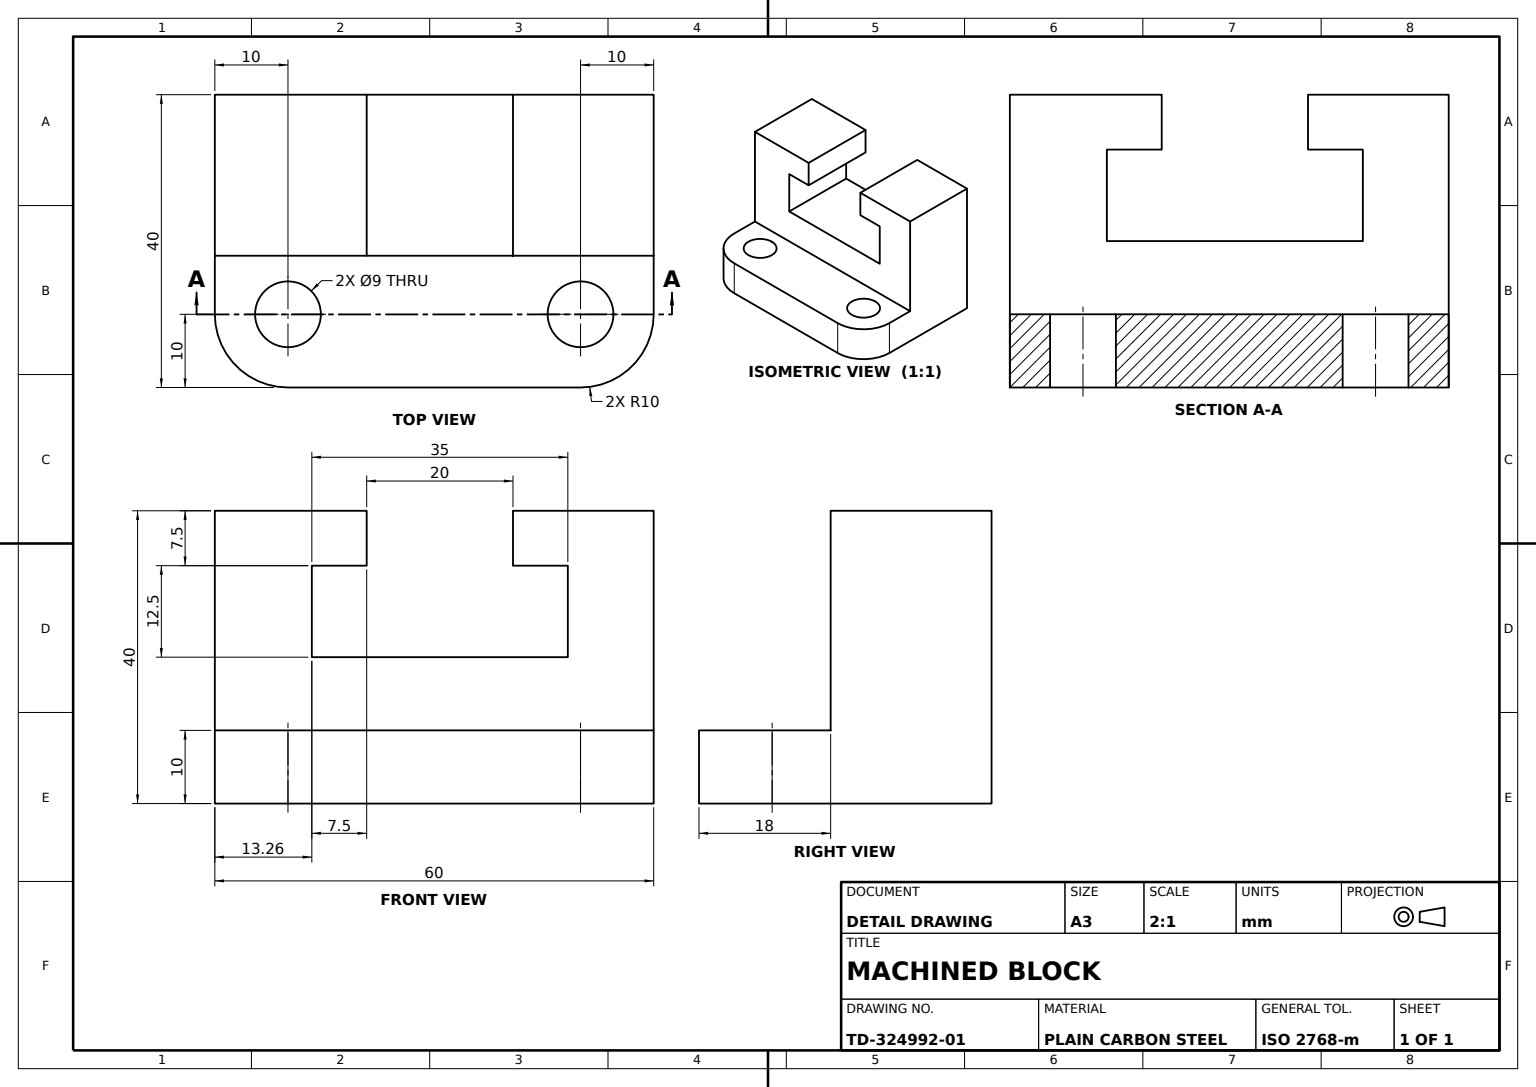
SolidWorks part; units mm, degrees
material "Plain Carbon Steel"
ref_plane "Front Plane" through (0, 0, 0) normal (0, 0, 1) x (1, 0, 0)
ref_plane "Top Plane" through (0, 0, 0) normal (0, 1, 0) x (1, 0, 0)
ref_plane "Right Plane" through (0, 0, 0) normal (1, 0, 0) x (0, 0, -1)
sketch "U-Bracket Profile Sketch" plane through (0, 0, 0) normal (0, 0, 1) x (1, 0, 0)
  line L0 (0, 0) -> (60, 0)
  line L1 (60, 0) -> (60, 40)
  line L2 (60, 40) -> (40.7619, 40)
  line L3 (40.7619, 40) -> (40.7619, 32.5)
  line L4 (40.7619, 32.5) -> (48.2619, 32.5)
  line L5 (48.2619, 32.5) -> (48.2619, 20)
  line L6 (48.2619, 20) -> (13.2619, 20)
  line L7 (13.2619, 20) -> (13.2619, 32.5)
  line L8 (20.7619, 32.5) -> (20.7619, 40)
  line L9 (20.7619, 40) -> (0, 40)
  line L10 (0, 40) -> (0, 0)
  line L11 (13.2619, 32.5) -> (20.7619, 32.5)
  point P12 (40.7619, 36.25)
  dimension "D1" = 60
  dimension "D2" = 40
  dimension "D3" = 20
  dimension "D4" = 35
  dimension "D5" = 7.5
  dimension "D6" = 7.5
  dimension "D7" = 12.5
  dimension "D8" = 12.5
  dimension "D9" = 7.5
  dimension "D10" = 13.2619
extrude "U-Bracket Body" add sketch "U-Bracket Profile Sketch" along normal blind 22
sketch "Base Plate Sketch" plane through (0, 0, 0) normal (0, -1, 0) x (1, 0, 0)
  line L0 (0, 22) -> (0, 30)
  line L1 (10, 40) -> (50, 40)
  line L2 (60, 30) -> (60, 22)
  line L7 (0, 0) -> (60, 0)
  line L8 (60, 0) -> (60, 22)
  line L9 (60, 22) -> (0, 22)
  line L10 (0, 22) -> (0, 0)
  line L11 (0, 0) -> (60, 0)
  line L12 (60, 0) -> (60, 22)
  line L14 (0, 22) -> (0, 0)
  arc A0 (60, 30) -> (50, 40) centre (50, 30) ccw
  arc A1 (10, 40) -> (0, 30) centre (10, 30) ccw
  point P9 (60, 40)
  dimension "D2" = 10
  dimension "D1" = 18
  dimension "D3" = 0
extrude "Base Plate" add sketch "Base Plate Sketch" against normal blind 10 contours L1 A0 L2 L12 L11 L14 L0 A1
sketch "Mounting Holes Sketch" plane through (0, 10, 0) normal (0, 1, 0) x (1, 0, 0)
  circle A0 centre (10, -30) radius 4.5
  circle A1 centre (50, -30) radius 4.5
  dimension "D1" = 9
  dimension "D2" = 9
extrude "Mounting Holes 2xØ9" cut sketch "Mounting Holes Sketch" against normal through all
